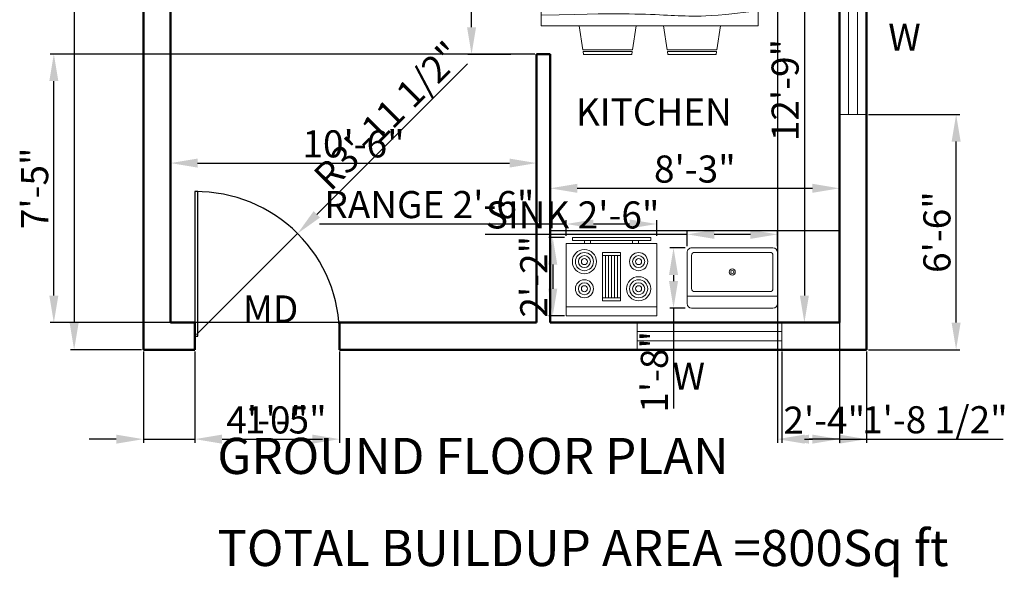
# Model space of a CAD drawing. Units: inches. Extents: x 1802 to 2621, y 1038 to 1686.
# Tile 1 of 5: x 1835 to 2161, y 1038 to 1223. Entities that reach past the tile are written whole.
import ezdxf

# ---------------------------------------------------------------- set-up
doc = ezdxf.new("R2010")
doc.units = ezdxf.units.IN
for name, color, linetype, lineweight in [('A-ANNO-DIMS', 2, 'Continuous', 18), ('A-ANNO-TEXT', 7, 'Continuous', 18), ('A-AREA-IDEN', 7, 'Continuous', 25), ('A-DOOR', 3, 'Continuous', 25), ('A-EQPM', 8, 'Continuous', 18), ('A-FLOR-CASE', 8, 'Continuous', 25), ('A-FLOR-FIXT', 9, 'Continuous', 18), ('A-FURN', 8, 'Continuous', 18), ('A-GLAZ', 4, 'Continuous', 18), ('A-WALL', 7, 'Continuous', 50)]:
    doc.layers.add(name, color=color, linetype=linetype, lineweight=lineweight)
doc.styles.get("Standard").update_dxf_attribs({"font": 'arial.ttf'})
doc.dimstyles.new('ISO-25', dxfattribs={"dimtxt": 9, "dimasz": 9, "dimexe": 1.25, "dimexo": 0.625, "dimtad": 1, "dimdec": 1, "dimrnd": 9, "dimlunit": 3, "dimtxsty": 'Standard', "dimcen": 2.5, "dimadec": 0, "dimazin": 0, "dimtfac": 1, "dimtdec": 1, "dimtmove": 0, "dimatfit": 3, "dimfxl": 1, "dimarcsym": 0})

# ---------------------------------------------------------------- blocks, each defined once
blk = doc.blocks.new('*D4')
at = {"layer": 'A-ANNO-DIMS', "color": 0, "lineweight": -2, "transparency": 16777216}
for p, q in [((1875.1, 1593.56), (1851.51, 1593.56)), ((1852.76, 1584.56), (1852.76, 1122.56)), ((1875.1, 1113.56), (1851.51, 1113.56))]:
    blk.add_line(p, q, dxfattribs=at)
at = {"layer": 'A-ANNO-DIMS', "color": 0, "transparency": 16777216}
for points in [[(1851.26, 1584.56), (1854.26, 1584.56), (1852.76, 1593.56)], [(1851.26, 1122.56), (1854.26, 1122.56), (1852.76, 1113.56)]]:
    blk.add_solid(points, dxfattribs=at)
at = {"layer": 'Defpoints', "color": 0, "transparency": 16777216}
for p in [(1875.73, 1593.56), (1852.76, 1113.56), (1875.73, 1113.56)]:
    blk.add_point(p, dxfattribs=at)
at = {"layer": 'A-ANNO-DIMS', "color": 0, "transparency": 16777216, "insert": (1847.54, 1353.56), "char_height": 9, "attachment_point": 5, "rotation": 90}
blk.add_mtext('39\'-9"', dxfattribs=at)
blk = doc.blocks.new('*D8')
at = {"layer": 'A-ANNO-DIMS', "color": 0, "lineweight": -2, "transparency": 16777216}
for p, q in [((2106.1, 1277.06), (2093.83, 1277.06)), ((2095.08, 1268.06), (2095.08, 1131.56)), ((2106.1, 1122.56), (2093.83, 1122.56))]:
    blk.add_line(p, q, dxfattribs=at)
at = {"layer": 'A-ANNO-DIMS', "color": 0, "transparency": 16777216}
for points in [[(2093.58, 1268.06), (2096.58, 1268.06), (2095.08, 1277.06)], [(2093.58, 1131.56), (2096.58, 1131.56), (2095.08, 1122.56)]]:
    blk.add_solid(points, dxfattribs=at)
at = {"layer": 'Defpoints', "color": 0, "transparency": 16777216}
for p in [(2106.73, 1277.06), (2095.08, 1122.56), (2106.73, 1122.56)]:
    blk.add_point(p, dxfattribs=at)
at = {"layer": 'A-ANNO-DIMS', "color": 0, "transparency": 16777216, "insert": (2089.86, 1199.81), "char_height": 9, "attachment_point": 5, "rotation": 90}
blk.add_mtext('12\'-9"', dxfattribs=at)
blk = doc.blocks.new('*D9')
at = {"layer": 'A-ANNO-DIMS', "color": 0, "lineweight": -2, "transparency": 16777216}
for p, q in [((2010.73, 1123.18), (2010.73, 1168.42)), ((2019.73, 1167.17), (2097.73, 1167.17)), ((2106.73, 1123.18), (2106.73, 1168.42))]:
    blk.add_line(p, q, dxfattribs=at)
at = {"layer": 'A-ANNO-DIMS', "color": 0, "transparency": 16777216}
for points in [[(2019.73, 1168.67), (2019.73, 1165.67), (2010.73, 1167.17)], [(2097.73, 1168.67), (2097.73, 1165.67), (2106.73, 1167.17)]]:
    blk.add_solid(points, dxfattribs=at)
at = {"layer": 'Defpoints', "color": 0, "transparency": 16777216}
for p in [(2106.73, 1167.17), (2010.73, 1122.56), (2106.73, 1122.56)]:
    blk.add_point(p, dxfattribs=at)
at = {"layer": 'A-ANNO-DIMS', "color": 0, "transparency": 16777216, "insert": (2058.73, 1172.4), "char_height": 9, "attachment_point": 5}
blk.add_mtext('8\'-3"', dxfattribs=at)
blk = doc.blocks.new('*D10')
at = {"layer": 'A-ANNO-DIMS', "color": 0, "lineweight": -2, "transparency": 16777216}
for p, q in [((1884.73, 1123.18), (1884.73, 1176.79)), ((2006.23, 1123.18), (2006.23, 1176.79)), ((1893.73, 1175.54), (1997.23, 1175.54))]:
    blk.add_line(p, q, dxfattribs=at)
at = {"layer": 'A-ANNO-DIMS', "color": 0, "transparency": 16777216}
for points in [[(1893.73, 1177.04), (1893.73, 1174.04), (1884.73, 1175.54)], [(1997.23, 1177.04), (1997.23, 1174.04), (2006.23, 1175.54)]]:
    blk.add_solid(points, dxfattribs=at)
at = {"layer": 'Defpoints', "color": 0, "transparency": 16777216}
for p in [(2006.23, 1175.54), (1884.73, 1122.56), (2006.23, 1122.56)]:
    blk.add_point(p, dxfattribs=at)
at = {"layer": 'A-ANNO-DIMS', "color": 0, "transparency": 16777216, "insert": (1945.48, 1180.76), "char_height": 9, "attachment_point": 5}
blk.add_mtext('10\'-6"', dxfattribs=at)
blk = doc.blocks.new('Dining Set - 36 x 72 in.')
for p, q in [((-22, 27.5), (-22.1562, 26.50042)), ((-5.8416, 26.5), (-22.1534, 26.5)), ((-22, 27.5), (-6, 27.5)), ((-5.8437, 26.49966), (-6, 27.5)), ((6, 27.5), (5.8438, 26.50042)), ((22.1584, 26.5), (5.8466, 26.5)), ((6, 27.5), (22, 27.5)), ((22.1563, 26.49966), (22, 27.5)), ((-22.2343, 26.00059), (-23.4847, 17.99762)), ((-22.2304, 26), (-5.7608, 26)), ((-4.5152, 17.99762), (-5.7655, 25.99926)), ((5.7657, 26.00059), (4.5153, 17.99762)), ((5.7696, 26), (22.2392, 26)), ((23.4848, 17.99762), (22.2345, 25.99926)), ((36, 18), (-36, 18)), ((-36, 18), (-36, -18)), ((36, -18), (36, 18)), ((-45.5, 8), (-44.5004, 8.15617)), ((-45.5, 8), (-45.5, -8)), ((-44.5, -8.15843), (-44.5, 8.15338)), ((-44.0006, 8.23428), (-35.9976, 9.48474)), ((-44, 8.23041), (-44, -8.23915)), ((44.0006, 8.23428), (35.9976, 9.48474)), ((44, 8.23041), (44, -8.23915)), ((44.5, -8.15843), (44.5, 8.15338)), ((45.5, 8), (44.5005, 8.15617)), ((45.5, 8), (45.5, -8)), ((-44.4997, -8.15631), (-45.5, -8)), ((-35.9976, -9.48476), (-43.9993, -8.2345)), ((35.9976, -9.48476), (43.9993, -8.2345)), ((44.4997, -8.15631), (45.5, -8)), ((-36, -18), (36, -18)), ((-22.2343, -26.0006), (-23.4847, -17.99762)), ((-4.5152, -17.99762), (-5.7655, -25.99928)), ((5.7657, -26.0006), (4.5153, -17.99762)), ((23.4848, -17.99762), (22.2345, -25.99928)), ((-22.2304, -26), (-5.7608, -26)), ((5.7696, -26), (22.2392, -26)), ((-22, -27.5), (-22.1562, -26.50044)), ((-5.8416, -26.5), (-22.1534, -26.5)), ((-22, -27.5), (-6, -27.5)), ((-5.8437, -26.49967), (-6, -27.5)), ((6, -27.5), (5.8438, -26.50044)), ((22.1584, -26.5), (5.8466, -26.5)), ((6, -27.5), (22, -27.5)), ((22.1563, -26.49967), (22, -27.5))]:
    blk.add_line(p, q)
for points in [[(-36, 15), (-31.1772, 14.97754), (-26.8079, 14.91406), (-22.8538, 14.81543), (-19.276, 14.6875), (-16.0362, 14.53613), (-13.0957, 14.36718), (-10.4159, 14.18652), (-7.9583, 14), (-5.6904, 13.81315), (-3.6035, 13.63021), (-1.6954, 13.45508), (0.0365, 13.29166), (1.5945, 13.14388), (2.9811, 13.01562), (4.1988, 12.9108), (5.25, 12.83333), (6.1393, 12.78613), (6.8802, 12.76823), (7.4883, 12.77767), (7.9792, 12.8125), (8.3685, 12.87077), (8.6719, 12.95052), (8.9049, 13.0498), (9.0833, 13.16666), (9.2205, 13.29899), (9.3216, 13.44401), (9.3895, 13.59879), (9.4271, 13.76041), (9.4373, 13.92594), (9.4232, 14.09245), (9.3875, 14.257), (9.3333, 14.41666), (9.2638, 14.56917), (9.1836, 14.71484), (9.0975, 14.85465), (9.0104, 14.98958), (8.9272, 15.1206), (8.8529, 15.2487), (8.7922, 15.37483), (8.75, 15.5), (8.7305, 15.62467), (8.7344, 15.74739), (8.7617, 15.86621), (8.8125, 15.97916), (8.8867, 16.08431), (8.9844, 16.17968), (9.1055, 16.26334), (9.25, 16.33333), (9.4189, 16.38802), (9.6172, 16.42708), (9.8506, 16.45052), (10.125, 16.45833), (10.4463, 16.45052), (10.8203, 16.42708), (11.2529, 16.38802), (11.75, 16.33333), (12.3184, 16.26318), (12.9694, 16.17838), (13.7151, 16.07991), (14.5677, 15.96875), (15.5395, 15.84586), (16.6426, 15.71224), (17.8893, 15.56884), (19.2917, 15.41666), (20.859, 15.25667), (22.5879, 15.08984), (24.4721, 14.91715), (26.5052, 14.73958), (28.6809, 14.5581), (30.9929, 14.3737), (33.4347, 14.18733), (36, 14)], [(-36, 10), (-28.9766, 10.14274), (-23.1725, 10.20442), (-18.4241, 10.19775), (-14.5677, 10.13541), (-11.4399, 10.03011), (-8.877, 9.89453), (-6.7154, 9.74137), (-4.7917, 9.58333), (-2.9698, 9.43082), (-1.2246, 9.28515), (0.4415, 9.14534), (2.026, 9.01041), (3.5266, 8.87939), (4.9408, 8.7513), (6.266, 8.62516), (7.5, 8.5), (8.6411, 8.37549), (9.6914, 8.2539), (10.6538, 8.13818), (11.5312, 8.03125), (12.3267, 7.93603), (13.043, 7.85547), (13.6831, 7.79248), (14.25, 7.75), (14.7471, 7.7303), (15.1797, 7.73307), (15.5537, 7.75732), (15.875, 7.80208), (16.1494, 7.86637), (16.3828, 7.94922), (16.5811, 8.04964), (16.75, 8.16666), (16.8944, 8.29915), (17.0143, 8.44531), (17.1089, 8.60319), (17.1771, 8.77083), (17.218, 8.94629), (17.2305, 9.1276), (17.2137, 9.31282), (17.1667, 9.5), (17.0895, 9.6875), (16.987, 9.875), (16.8649, 10.0625), (16.7292, 10.25), (16.5856, 10.4375), (16.4401, 10.625), (16.2985, 10.8125), (16.1667, 11), (16.05, 11.18733), (15.9518, 11.3737), (15.8752, 11.5581), (15.8229, 11.73958), (15.798, 11.91715), (15.8034, 12.08984), (15.842, 12.25667), (15.9167, 12.41666), (16.0295, 12.56836), (16.1784, 12.70833), (16.3605, 12.83268), (16.5729, 12.9375), (16.8127, 13.01888), (17.0768, 13.07291), (17.3625, 13.0957), (17.6667, 13.08333), (17.9894, 13.03312), (18.3418, 12.94726), (18.7382, 12.82918), (19.1927, 12.68229), (19.7195, 12.51001), (20.3327, 12.31575), (21.0465, 12.10294), (21.875, 11.875), (22.8357, 11.63354), (23.959, 11.37304), (25.2786, 11.08618), (26.8282, 10.76562), (28.6414, 10.40405), (30.752, 9.99414), (33.1936, 9.52856), (36, 9)], [(-36, 5.5), (-30.7157, 5.3348), (-26.069, 5.20963), (-21.9946, 5.11767), (-18.4271, 5.05208), (-15.3009, 5.00602), (-12.5508, 4.97265), (-10.1112, 4.94515), (-7.9167, 4.91666), (-5.909, 4.88167), (-4.0586, 4.83984), (-2.3429, 4.79215), (-0.7396, 4.73958), (0.7739, 4.6831), (2.22, 4.6237), (3.6213, 4.56233), (5, 4.5), (6.373, 4.43782), (7.7344, 4.3776), (9.0723, 4.32129), (10.375, 4.27083), (11.6309, 4.22819), (12.8281, 4.19531), (13.9551, 4.17415), (15, 4.16666), (15.954, 4.17448), (16.819, 4.19791), (17.6001, 4.23698), (18.3021, 4.29166), (18.9299, 4.36198), (19.4883, 4.44791), (19.9823, 4.54948), (20.4167, 4.66666), (20.7969, 4.79899), (21.1302, 4.94401), (21.4245, 5.09879), (21.6875, 5.26041), (21.9271, 5.42594), (22.1511, 5.59245), (22.3672, 5.757), (22.5834, 5.91666), (22.8065, 6.06868), (23.0404, 6.21093), (23.2879, 6.34147), (23.5521, 6.45833), (23.8358, 6.55957), (24.142, 6.64323), (24.4735, 6.70735), (24.8334, 6.75), (25.2235, 6.76969), (25.642, 6.76692), (26.0858, 6.74267), (26.5521, 6.69791), (27.0379, 6.63362), (27.5404, 6.55078), (28.0565, 6.45036), (28.5834, 6.33333), (29.1242, 6.19987), (29.7071, 6.04687), (30.3661, 5.87044), (31.1354, 5.66666), (32.0493, 5.43164), (33.142, 5.16146), (34.4475, 4.85221), (36, 4.5)], [(-36, -1), (-30.7915, -0.6591), (-26.0195, -0.38216), (-21.6519, -0.16284), (-17.6563, 0.00521), (-14.0005, 0.12833), (-10.6523, 0.21289), (-7.5796, 0.26522), (-4.75, 0.29166), (-2.134, 0.29793), (0.2878, 0.28711), (2.5317, 0.26163), (4.6146, 0.22396), (6.5529, 0.17651), (8.3633, 0.12174), (10.0623, 0.06209), (11.6667, 0), (13.1899, -0.06201), (14.6341, -0.1211), (15.9982, -0.17432), (17.2813, -0.21875), (18.4823, -0.25147), (19.6003, -0.26953), (20.6343, -0.27002), (21.5834, -0.25), (22.4481, -0.20768), (23.2357, -0.14584), (23.9549, -0.06836), (24.6146, 0.02083), (25.2235, 0.11784), (25.7904, 0.21875), (26.3241, 0.31966), (26.8334, 0.41666), (27.3265, 0.50618), (27.8099, 0.58593), (28.2894, 0.65397), (28.7709, 0.70833), (29.2601, 0.74707), (29.763, 0.76823), (30.2855, 0.76985), (30.8334, 0.75), (31.4088, 0.70784), (31.9994, 0.64713), (32.589, 0.57275), (33.1615, 0.48958), (33.7008, 0.4025), (34.1908, 0.3164), (34.6153, 0.23616), (34.9584, 0.16666), (35.2099, 0.11165), (35.3848, 0.07031), (35.504, 0.04069), (35.5886, 0.02083), (35.6594, 0.00879), (35.7377, 0.0026), (35.8442, 0.00032), (36, 0)], [(-36, -6.5), (-27.1843, -6.31267), (-20.084, -6.1263), (-14.469, -5.9419), (-10.1094, -5.76042), (-6.7752, -5.58285), (-4.2363, -5.41016), (-2.2629, -5.24333), (-0.625, -5.08334), (0.8708, -4.93099), (2.2715, -4.78646), (3.5872, -4.64974), (4.8281, -4.52084), (6.0046, -4.39974), (7.127, -4.28646), (8.2053, -4.18099), (9.25, -4.08334), (10.2705, -3.99382), (11.2734, -3.91407), (12.2647, -3.84603), (13.25, -3.79167), (14.2354, -3.75293), (15.2266, -3.73177), (16.2295, -3.73015), (17.25, -3.75), (18.2912, -3.79248), (19.3451, -3.85547), (20.4009, -3.93604), (21.4479, -4.03125), (22.4754, -4.13819), (23.4727, -4.25391), (24.4289, -4.37549), (25.3334, -4.5), (26.1785, -4.62492), (26.9694, -4.74935), (27.7145, -4.87281), (28.4219, -4.99479), (29.1, -5.11483), (29.7572, -5.23242), (30.4016, -5.34709), (31.0417, -5.45834), (31.6837, -5.56437), (32.3262, -5.65821), (32.9658, -5.73153), (33.599, -5.77604), (34.2224, -5.78345), (34.8327, -5.74545), (35.4264, -5.65373), (36, -5.5)], [(-36, -10), (-26.4022, -9.81299), (-18.4675, -9.62891), (-11.9839, -9.45069), (-6.7396, -9.28125), (-2.5226, -9.12354), (0.8789, -8.98047), (3.6769, -8.85498), (6.0833, -8.75), (8.2767, -8.66765), (10.3021, -8.60677), (12.1712, -8.56543), (13.8958, -8.54167), (15.4876, -8.53353), (16.9583, -8.53907), (18.3197, -8.55632), (19.5834, -8.58334), (20.7616, -8.61841), (21.8685, -8.66081), (22.9188, -8.71004), (23.9271, -8.76563), (24.9081, -8.82707), (25.8763, -8.89388), (26.8465, -8.96558), (27.8334, -9.04167), (28.8474, -9.12118), (29.8828, -9.20117), (30.93, -9.27824), (31.9792, -9.34896), (33.0205, -9.40991), (34.0443, -9.45768), (35.0407, -9.48885), (36, -9.5)], [(-36, -14.5), (-30.0881, -14.33513), (-25.0332, -14.21224), (-20.7312, -14.12647), (-17.0781, -14.07292), (-13.97, -14.04671), (-11.3027, -14.04297), (-8.9724, -14.05681), (-6.875, -14.08334), (-4.9224, -14.11833), (-3.0905, -14.16016), (-1.3709, -14.20785), (0.2448, -14.26042), (1.7647, -14.3169), (3.1973, -14.3763), (4.5507, -14.43767), (5.8333, -14.5), (7.0554, -14.5621), (8.235, -14.62175), (9.3922, -14.67652), (10.5469, -14.72396), (11.7192, -14.76164), (12.929, -14.78711), (14.1965, -14.79794), (15.5417, -14.79167), (16.9933, -14.76424), (18.6152, -14.70508), (20.4804, -14.60197), (22.6615, -14.44271), (25.2312, -14.21509), (28.2624, -13.9069), (31.8277, -13.50594), (36, -13)]]:
    blk.add_lwpolyline(points)
blk = doc.blocks.new('Range-Oven - 30 in top')
for p, q in [((0, -3), (30, -3)), ((12, -6), (18, -6)), ((13, -20), (13, -6)), ((14, -6), (14, -20)), ((15, -20), (15, -6)), ((16, -6), (16, -20)), ((17, -20), (17, -6)), ((18, -20), (12, -20)), ((6, -24), (6, -25)), ((8, -25), (8, -24)), ((22, -25), (22, -24)), ((24, -24), (24, -25))]:
    blk.add_line(p, q)
for points in [[(0, -24), (0, 0), (30, 0), (30, -24)], [(12, -21), (12, -5), (18, -5), (18, -21)], [(2, -26), (2, -25), (28, -25), (28, -26)]]:
    blk.add_lwpolyline(points, close=True)
for centre, radius in [((6, -9), 4), ((6, -9), 3), ((24, -9), 3), ((6, -9), 2), ((6, -9), 1), ((24, -9), 2), ((24, -9), 1), ((6, -18), 3), ((6, -18), 2), ((24, -18), 4), ((24, -18), 3), ((24, -18), 2), ((6, -18), 1), ((24, -18), 1)]:
    blk.add_circle(centre, radius)
blk = doc.blocks.new('Sink-single - 30 in top')
blk.add_line((-15, -3.999996), (15, -3.999996))
for points in [[(-13.5, 0), (13.5, 0)], [(-15, -18.499996), (-15, -1.5)], [(15, -1.5), (15, -18.499996)], [(-13.5, -17.499996), (-13.5, -6.499996)], [(-12.5, -5.499996), (12.5, -5.499996)], [(13.5, -6.499996), (13.5, -17.499996)], [(12.5, -18.499996), (-12.5, -18.499996)], [(13.5, -19.999996), (-13.5, -19.999996)]]:
    blk.add_lwpolyline(points)
for radius in [1, 0.5]:
    blk.add_circle((0, -11.999996), radius)
for centre, radius, start, end in [((-13.5, -1.5), 1.5, 90, 180), ((13.5, -1.5), 1.5, 0, 90), ((-12.5, -6.499996), 1, 90, 180), ((12.5, -6.499996), 1, 0, 90), ((-13.5, -18.499996), 1.5, 180, 270), ((-12.5, -17.499996), 1, 180, 270), ((12.5, -17.499996), 1, 270, 0), ((13.5, -18.499996), 1.5, 270, 0)]:
    blk.add_arc(centre, radius, start, end)
blk = doc.blocks.new('WIN-48IN')
for p, q in [((9, 48), (0, 48)), ((3, 48), (3, 0)), ((6, 48), (6, 0)), ((9, 0), (0, 0))]:
    blk.add_line(p, q)
blk = doc.blocks.new('*D60')
at = {"layer": 'A-ANNO-DIMS', "color": 0, "lineweight": -2, "transparency": 16777216}
for p, q in [((1997.66, 1266.65), (1983.38, 1266.65)), ((1984.63, 1220.65), (1984.63, 1257.65)), ((1997.66, 1211.65), (1983.38, 1211.65))]:
    blk.add_line(p, q, dxfattribs=at)
at = {"layer": 'A-ANNO-DIMS', "color": 0, "transparency": 16777216}
for points in [[(1983.13, 1257.65), (1986.13, 1257.65), (1984.63, 1266.65)], [(1983.13, 1220.65), (1986.13, 1220.65), (1984.63, 1211.65)]]:
    blk.add_solid(points, dxfattribs=at)
at = {"layer": 'Defpoints', "color": 0, "transparency": 16777216}
for p in [(1984.63, 1266.65), (1998.28, 1266.65), (1998.28, 1211.65)]:
    blk.add_point(p, dxfattribs=at)
at = {"layer": 'A-ANNO-DIMS', "color": 0, "transparency": 16777216, "insert": (1979.51, 1239.15), "char_height": 9, "attachment_point": 5, "rotation": 90}
blk.add_mtext('4\'-7"', dxfattribs=at)
blk = doc.blocks.new('*D61')
at = {"layer": 'A-ANNO-DIMS', "color": 0, "lineweight": -2, "transparency": 16777216}
for p, q in [((2016.08, 1155.31), (1934.17, 1155.31)), ((2016.08, 1151.43), (2016.08, 1156.56)), ((2037.08, 1155.31), (2025.08, 1155.31)), ((2046.08, 1151.43), (2046.08, 1156.56))]:
    blk.add_line(p, q, dxfattribs=at)
at = {"layer": 'A-ANNO-DIMS', "color": 0, "transparency": 16777216}
for points in [[(2025.08, 1156.81), (2025.08, 1153.81), (2016.08, 1155.31)], [(2037.08, 1156.81), (2037.08, 1153.81), (2046.08, 1155.31)]]:
    blk.add_solid(points, dxfattribs=at)
at = {"layer": 'Defpoints', "color": 0, "transparency": 16777216}
for p in [(2016.08, 1155.31), (2016.08, 1150.81), (2046.08, 1150.81)]:
    blk.add_point(p, dxfattribs=at)
at = {"layer": 'A-ANNO-DIMS', "color": 0, "transparency": 16777216, "insert": (1970.63, 1160.59), "char_height": 9, "attachment_point": 5}
blk.add_mtext('RANGE 2\'-6"', dxfattribs=at)
blk = doc.blocks.new('*D62')
at = {"layer": 'A-ANNO-DIMS', "color": 0, "lineweight": -2, "transparency": 16777216}
for p, q in [((2015.46, 1150.81), (2010.33, 1150.81)), ((2011.58, 1141.81), (2011.58, 1133.81)), ((2015.46, 1124.81), (2010.33, 1124.81))]:
    blk.add_line(p, q, dxfattribs=at)
at = {"layer": 'A-ANNO-DIMS', "color": 0, "transparency": 16777216}
for points in [[(2010.08, 1141.81), (2013.08, 1141.81), (2011.58, 1150.81)], [(2010.08, 1133.81), (2013.08, 1133.81), (2011.58, 1124.81)]]:
    blk.add_solid(points, dxfattribs=at)
at = {"layer": 'Defpoints', "color": 0, "transparency": 16777216}
for p in [(2016.08, 1150.81), (2011.58, 1124.81), (2016.08, 1124.81)]:
    blk.add_point(p, dxfattribs=at)
at = {"layer": 'A-ANNO-DIMS', "color": 0, "transparency": 16777216, "insert": (2006.44, 1137.81), "char_height": 9, "attachment_point": 5, "rotation": 90}
blk.add_mtext('2\'-2"', dxfattribs=at)
blk = doc.blocks.new('*D63')
at = {"layer": 'A-ANNO-DIMS', "color": 0, "lineweight": -2, "transparency": 16777216}
for p, q in [((2056.16, 1151.87), (1989.19, 1151.87)), ((2056.16, 1148), (2056.16, 1153.12)), ((2077.16, 1151.87), (2065.16, 1151.87)), ((2086.16, 1148), (2086.16, 1153.12))]:
    blk.add_line(p, q, dxfattribs=at)
at = {"layer": 'A-ANNO-DIMS', "color": 0, "transparency": 16777216}
for points in [[(2065.16, 1153.37), (2065.16, 1150.37), (2056.16, 1151.87)], [(2077.16, 1153.37), (2077.16, 1150.37), (2086.16, 1151.87)]]:
    blk.add_solid(points, dxfattribs=at)
at = {"layer": 'Defpoints', "color": 0, "transparency": 16777216}
for p in [(2056.16, 1151.87), (2056.16, 1147.37), (2086.16, 1147.37)]:
    blk.add_point(p, dxfattribs=at)
at = {"layer": 'A-ANNO-DIMS', "color": 0, "transparency": 16777216, "insert": (2018.18, 1157.15), "char_height": 9, "attachment_point": 5}
blk.add_mtext('SINK 2\'-6"', dxfattribs=at)
blk = doc.blocks.new('*D64')
at = {"layer": 'A-ANNO-DIMS', "color": 0, "lineweight": -2, "transparency": 16777216}
for p, q in [((2055.54, 1147.37), (2050.41, 1147.37)), ((2051.66, 1138.37), (2051.66, 1136.37)), ((2055.54, 1127.37), (2050.41, 1127.37)), ((2051.66, 1127.37), (2051.66, 1094.05))]:
    blk.add_line(p, q, dxfattribs=at)
at = {"layer": 'A-ANNO-DIMS', "color": 0, "transparency": 16777216}
for points in [[(2050.16, 1138.37), (2053.16, 1138.37), (2051.66, 1147.37)], [(2050.16, 1136.37), (2053.16, 1136.37), (2051.66, 1127.37)]]:
    blk.add_solid(points, dxfattribs=at)
at = {"layer": 'Defpoints', "color": 0, "transparency": 16777216}
for p in [(2056.16, 1147.37), (2051.66, 1127.37), (2056.16, 1127.37)]:
    blk.add_point(p, dxfattribs=at)
at = {"layer": 'A-ANNO-DIMS', "color": 0, "transparency": 16777216, "insert": (2046.44, 1106.21), "char_height": 9, "attachment_point": 5, "rotation": 90}
blk.add_mtext('1\'-8"', dxfattribs=at)
blk = doc.blocks.new('*D65')
at = {"layer": 'A-ANNO-DIMS', "color": 0, "lineweight": -2, "transparency": 16777216}
for p, q in [((1875.73, 1112.93), (1875.73, 1082.61)), ((1892.83, 1112.93), (1892.83, 1082.61)), ((1866.73, 1083.86), (1857.73, 1083.86)), ((1875.73, 1083.86), (1892.83, 1083.86)), ((1901.83, 1083.86), (1935.16, 1083.86))]:
    blk.add_line(p, q, dxfattribs=at)
at = {"layer": 'A-ANNO-DIMS', "color": 0, "transparency": 16777216}
for points in [[(1866.73, 1085.36), (1866.73, 1082.36), (1875.73, 1083.86)], [(1901.83, 1085.36), (1901.83, 1082.36), (1892.83, 1083.86)]]:
    blk.add_solid(points, dxfattribs=at)
at = {"layer": 'Defpoints', "color": 0, "transparency": 16777216}
for p in [(1875.73, 1113.56), (1892.83, 1113.56), (1892.83, 1083.86)]:
    blk.add_point(p, dxfattribs=at)
at = {"layer": 'A-ANNO-DIMS', "color": 0, "transparency": 16777216, "insert": (1922.99, 1089.08), "char_height": 9, "attachment_point": 5}
blk.add_mtext('1\'-5"', dxfattribs=at)
blk = doc.blocks.new('*D72')
at = {"layer": 'A-ANNO-DIMS', "color": 0, "lineweight": -2, "transparency": 16777216}
for p, q in [((2116.35, 1191.68), (2146.68, 1191.68)), ((2145.43, 1122.56), (2145.43, 1182.68)), ((2116.35, 1113.56), (2146.68, 1113.56))]:
    blk.add_line(p, q, dxfattribs=at)
at = {"layer": 'A-ANNO-DIMS', "color": 0, "transparency": 16777216}
for points in [[(2143.93, 1182.68), (2146.93, 1182.68), (2145.43, 1191.68)], [(2143.93, 1122.56), (2146.93, 1122.56), (2145.43, 1113.56)]]:
    blk.add_solid(points, dxfattribs=at)
at = {"layer": 'Defpoints', "color": 0, "transparency": 16777216}
for p in [(2115.73, 1191.68), (2145.43, 1191.68), (2115.73, 1113.56)]:
    blk.add_point(p, dxfattribs=at)
at = {"layer": 'A-ANNO-DIMS', "color": 0, "transparency": 16777216, "insert": (2140.21, 1152.62), "char_height": 9, "attachment_point": 5, "rotation": 90}
blk.add_mtext('6\'-6"', dxfattribs=at)
blk = doc.blocks.new('*D73')
at = {"layer": 'A-ANNO-DIMS', "color": 0, "lineweight": -2, "transparency": 16777216}
for p, q in [((2087.63, 1112.93), (2087.63, 1082.61)), ((2115.73, 1112.93), (2115.73, 1082.61)), ((2106.73, 1083.86), (2096.63, 1083.86))]:
    blk.add_line(p, q, dxfattribs=at)
at = {"layer": 'A-ANNO-DIMS', "color": 0, "transparency": 16777216}
for points in [[(2096.63, 1085.36), (2096.63, 1082.36), (2087.63, 1083.86)], [(2106.73, 1085.36), (2106.73, 1082.36), (2115.73, 1083.86)]]:
    blk.add_solid(points, dxfattribs=at)
at = {"layer": 'Defpoints', "color": 0, "transparency": 16777216}
for p in [(2087.63, 1113.56), (2115.73, 1113.56), (2087.63, 1083.86)]:
    blk.add_point(p, dxfattribs=at)
at = {"layer": 'A-ANNO-DIMS', "color": 0, "transparency": 16777216, "insert": (2101.68, 1089), "char_height": 9, "attachment_point": 5}
blk.add_mtext('2\'-4"', dxfattribs=at)
blk = doc.blocks.new('*D74')
at = {"layer": 'A-ANNO-DIMS', "color": 0, "lineweight": -2, "transparency": 16777216}
for p, q in [((1892.83, 1112.93), (1892.83, 1082.61)), ((1940.83, 1112.93), (1940.83, 1082.61)), ((1901.83, 1083.86), (1931.83, 1083.86))]:
    blk.add_line(p, q, dxfattribs=at)
at = {"layer": 'A-ANNO-DIMS', "color": 0, "transparency": 16777216}
for points in [[(1901.83, 1085.36), (1901.83, 1082.36), (1892.83, 1083.86)], [(1931.83, 1085.36), (1931.83, 1082.36), (1940.83, 1083.86)]]:
    blk.add_solid(points, dxfattribs=at)
at = {"layer": 'Defpoints', "color": 0, "transparency": 16777216}
for p in [(1892.83, 1113.56), (1940.83, 1113.56), (1940.83, 1083.86)]:
    blk.add_point(p, dxfattribs=at)
at = {"layer": 'A-ANNO-DIMS', "color": 0, "transparency": 16777216, "insert": (1916.83, 1089.08), "char_height": 9, "attachment_point": 5}
blk.add_mtext('4\'-0"', dxfattribs=at)
blk = doc.blocks.new('*D75')
at = {"layer": 'A-ANNO-DIMS', "color": 0, "lineweight": -2, "transparency": 16777216}
for p, q in [((2086.14, 1280.93), (2086.14, 1082.61)), ((2106.73, 1278.98), (2106.73, 1082.61)), ((2095.14, 1083.86), (2097.73, 1083.86)), ((2106.73, 1083.86), (2161.03, 1083.86))]:
    blk.add_line(p, q, dxfattribs=at)
at = {"layer": 'A-ANNO-DIMS', "color": 0, "transparency": 16777216}
for points in [[(2095.14, 1085.36), (2095.14, 1082.36), (2086.14, 1083.86)], [(2097.73, 1085.36), (2097.73, 1082.36), (2106.73, 1083.86)]]:
    blk.add_solid(points, dxfattribs=at)
at = {"layer": 'Defpoints', "color": 0, "transparency": 16777216}
for p in [(2086.14, 1281.56), (2106.73, 1279.61), (2106.73, 1083.86)]:
    blk.add_point(p, dxfattribs=at)
at = {"layer": 'A-ANNO-DIMS', "color": 0, "transparency": 16777216, "insert": (2138.38, 1089.14), "char_height": 9, "attachment_point": 5}
blk.add_mtext('1\'-8 1/2"', dxfattribs=at)
blk = doc.blocks.new('*D77')
at = {"layer": 'A-ANNO-DIMS', "color": 0, "lineweight": -2, "transparency": 16777216}
for p, q in [((2005.6, 1211.75), (1844.78, 1211.75)), ((1846.03, 1131.56), (1846.03, 1202.75)), ((2005.6, 1122.56), (1844.78, 1122.56))]:
    blk.add_line(p, q, dxfattribs=at)
at = {"layer": 'A-ANNO-DIMS', "color": 0, "transparency": 16777216}
for points in [[(1844.53, 1202.75), (1847.53, 1202.75), (1846.03, 1211.75)], [(1844.53, 1131.56), (1847.53, 1131.56), (1846.03, 1122.56)]]:
    blk.add_solid(points, dxfattribs=at)
at = {"layer": 'Defpoints', "color": 0, "transparency": 16777216}
for p in [(1846.03, 1211.75), (2006.23, 1211.75), (2006.23, 1122.56)]:
    blk.add_point(p, dxfattribs=at)
at = {"layer": 'A-ANNO-DIMS', "color": 0, "transparency": 16777216, "insert": (1840.83, 1167.15), "char_height": 9, "attachment_point": 5, "rotation": 90}
blk.add_mtext('7\'-5"', dxfattribs=at)
blk = doc.blocks.new('*D78')
at = {"layer": 'A-ANNO-DIMS', "color": 0, "lineweight": -2, "transparency": 16777216}
for p, q in [((1983.31, 1208.54), (1933.28, 1158.51)), ((1893.33, 1118.56), (1926.92, 1152.15))]:
    blk.add_line(p, q, dxfattribs=at)
at = {"layer": 'A-ANNO-DIMS', "color": 0, "transparency": 16777216}
blk.add_solid([(1932.22, 1159.57), (1934.34, 1157.45), (1926.92, 1152.15)], dxfattribs=at)
at = {"layer": 'Defpoints', "color": 0, "transparency": 16777216}
for p in [(1926.92, 1152.15), (1893.33, 1118.56)]:
    blk.add_point(p, dxfattribs=at)
at = {"layer": 'A-ANNO-DIMS', "color": 0, "transparency": 16777216, "insert": (1957.74, 1190.44), "char_height": 9, "attachment_point": 5, "rotation": 45}
blk.add_mtext('R3\'-11 1/2"', dxfattribs=at)

msp = doc.modelspace()

# ---------------------------------------------------------------- linework, layer by layer
at = {"layer": 'A-DOOR'}
for p, q in [((1893.83, 1166.06), (1892.83, 1166.06)), ((1892.83, 1166.06), (1892.83, 1122.56)), ((1893.83, 1118.06), (1893.83, 1166.06)), ((1892.83, 1118.06), (1893.83, 1118.06))]:
    msp.add_line(p, q, dxfattribs=at)
msp.add_arc((1893.33, 1118.56), 47.5, 359.3969, 90.6031, dxfattribs=at)
at = {"layer": 'A-FLOR-CASE'}
msp.add_line((2010.73, 1153.18), (2106.73, 1153.18), dxfattribs=at)
at = {"layer": 'A-WALL'}
for p, q in [((1875.73, 1593.56), (1875.73, 1113.56)), ((2115.73, 1113.56), (2115.73, 1593.56)), ((1884.73, 1341.56), (1884.73, 1122.56)), ((2106.73, 1122.56), (2106.73, 1341.56)), ((2006.23, 1122.56), (2006.23, 1211.75)), ((2010.73, 1211.75), (2006.23, 1211.75)), ((2010.73, 1122.56), (2010.73, 1211.75)), ((1884.73, 1122.56), (1892.83, 1122.56)), ((1892.83, 1122.56), (1892.83, 1113.56)), ((1940.83, 1122.56), (1940.83, 1113.56)), ((1940.83, 1122.56), (2006.23, 1122.56)), ((2010.73, 1122.56), (2106.73, 1122.56)), ((1875.73, 1113.56), (1892.83, 1113.56)), ((1940.83, 1113.56), (2115.73, 1113.56))]:
    msp.add_line(p, q, dxfattribs=at)

# ---------------------------------------------------------------- block references
at = {"layer": 'A-EQPM', "rotation": 180}
msp.add_blockref('Range-Oven - 30 in top', (2046.08, 1124.81), dxfattribs=at)
at = {"layer": 'A-FLOR-FIXT', "rotation": 180}
msp.add_blockref('Sink-single - 30 in top', (2071.16, 1127.37), dxfattribs=at)
at = {"layer": 'A-FURN'}
msp.add_blockref('Dining Set - 36 x 72 in.', (2043.78, 1239.15), dxfattribs=at)
at = {"layer": 'A-GLAZ'}
for p, rotation in [((2115.73, 1239.68), 180), ((2039.63, 1122.56), 270.0000000000002)]:
    msp.add_blockref('WIN-48IN', p, dxfattribs=dict(at, rotation=rotation))

# ---------------------------------------------------------------- texts
at = {"layer": 'A-ANNO-TEXT', "attachment_point": 1}
for s, width, insert, char_height in [('W', 30.0361, (2122.91, 1221.84), 9), ('MD ', 17.1074, (1908.74, 1131.6), 9), ('W', 30.0361, (2051.33, 1109.3), 9), ('GROUND FLOOR PLAN', 217.7869, (1900.28, 1084.29), 12)]:
    msp.add_mtext_dynamic_manual_height_columns(s, width=width, gutter_width=12.5, heights=[0], dxfattribs=dict(at, insert=insert, char_height=char_height))
at = {"layer": 'A-AREA-IDEN', "attachment_point": 1}
for s, width, insert, char_height in [('KITCHEN', 82.6611, (2019.24, 1197.01), 9), ('TOTAL BUILDUP AREA =800Sq ft', 272.6952, (1900.28, 1053.72), 12)]:
    msp.add_mtext_dynamic_manual_height_columns(s, width=width, gutter_width=12.5, heights=[0], dxfattribs=dict(at, insert=insert, char_height=char_height))

# ---------------------------------------------------------------- dimensions: what is measured, and where the dimension line sits
at = {"layer": 'A-ANNO-DIMS'}
for base, p1, p2, angle, override, picture, middle in [((1852.76, 1113.56), (1875.73, 1593.56), (1875.73, 1113.56), 90, {"dimclrd": 0, "dimclre": 0, "dimclrt": 0}, '*D4', (1847.54, 1353.56)), ((2095.08, 1122.56), (2106.73, 1277.06), (2106.73, 1122.56), 90, {"dimclrd": 0, "dimclre": 0, "dimclrt": 0}, '*D8', (2089.86, 1199.81)), ((1984.63, 1266.65), (1998.28, 1211.65), (1998.28, 1266.65), 90, {"dimdec": 1, "dimlfac": 1, "dimrnd": 0, "dimzin": 1, "dimdsep": 46, "dimlunit": 4, "dimfrac": 2}, '*D60', (1979.51, 1239.15)), ((1846.03, 1211.75), (2006.23, 1122.56), (2006.23, 1211.75), 90, {"dimdec": 1, "dimlfac": 1, "dimrnd": 0, "dimzin": 1, "dimdsep": 46, "dimlunit": 4, "dimfrac": 2}, '*D77', (1840.83, 1167.15)), ((2145.43, 1191.68), (2115.73, 1113.56), (2115.73, 1191.68), 90, {"dimdec": 1, "dimlfac": 1, "dimrnd": 0, "dimzin": 1, "dimdsep": 46, "dimlunit": 4, "dimfrac": 2}, '*D72', (2140.21, 1152.62)), ((2011.58, 1124.81), (2016.08, 1150.81), (2016.08, 1124.81), 270, {"dimdec": 1, "dimlfac": 1, "dimrnd": 0, "dimzin": 1, "dimdsep": 46, "dimlunit": 4, "dimfrac": 2}, '*D62', (2006.44, 1137.81)), ((2051.66, 1127.37), (2056.16, 1147.37), (2056.16, 1127.37), 270, {"dimdec": 1, "dimlfac": 1, "dimrnd": 0, "dimzin": 1, "dimdsep": 46, "dimlunit": 4, "dimfrac": 2}, '*D64', (2046.44, 1106.21))]:
    dim = msp.add_linear_dim(base=base, p1=p1, p2=p2, angle=angle, dimstyle='ISO-25', override=override, dxfattribs=at)
    dim.commit()
    dim.dimension.update_dxf_attribs({"geometry": picture, "text_midpoint": middle})
for base, p1, p2, override, picture, middle in [((2106.73, 1083.86), (2086.14, 1281.56), (2106.73, 1279.61), {"dimdec": 1, "dimlfac": 1, "dimrnd": 0, "dimzin": 1, "dimdsep": 46, "dimlunit": 4, "dimfrac": 2}, '*D75', (2138.38, 1089.14)), ((2006.23, 1175.54), (1884.73, 1122.56), (2006.23, 1122.56), {"dimclrd": 0, "dimclre": 0, "dimclrt": 0}, '*D10', (1945.48, 1180.76)), ((2106.73, 1167.17), (2010.73, 1122.56), (2106.73, 1122.56), {"dimclrd": 0, "dimclre": 0, "dimclrt": 0}, '*D9', (2058.73, 1172.4)), ((1892.83, 1083.86), (1875.73, 1113.56), (1892.83, 1113.56), {"dimdec": 1, "dimlfac": 1, "dimrnd": 0, "dimzin": 1, "dimdsep": 46, "dimlunit": 4, "dimfrac": 2}, '*D65', (1922.99, 1089.08)), ((1940.83, 1083.86), (1892.83, 1113.56), (1940.83, 1113.56), {"dimdec": 1, "dimlfac": 1, "dimrnd": 0, "dimzin": 1, "dimdsep": 46, "dimlunit": 4, "dimfrac": 2}, '*D74', (1916.83, 1089.08)), ((2087.63, 1083.86), (2115.73, 1113.56), (2087.63, 1113.56), {"dimdec": 1, "dimlfac": 1, "dimrnd": 0, "dimzin": 1, "dimdsep": 46, "dimlunit": 4, "dimfrac": 2}, '*D73', (2101.68, 1089))]:
    dim = msp.add_linear_dim(base=base, p1=p1, p2=p2, dimstyle='ISO-25', override=override, dxfattribs=at)
    dim.commit()
    dim.dimension.update_dxf_attribs({"geometry": picture, "text_midpoint": middle})
dim = msp.add_radius_dim(center=(1893.33, 1118.56), mpoint=(1926.92, 1152.15), dimstyle='ISO-25', override={"dimdec": 1, "dimlfac": 1, "dimrnd": 0, "dimzin": 1, "dimdsep": 46, "dimlunit": 4, "dimfrac": 2}, dxfattribs=at)
dim.commit()
dim.dimension.update_dxf_attribs({"geometry": '*D78', "text_midpoint": (1957.74, 1190.44)})
for base, p1, p2, text, picture, middle in [((2016.08, 1155.31), (2046.08, 1150.81), (2016.08, 1150.81), 'RANGE <>', '*D61', (1970.63, 1160.59)), ((2056.16, 1151.87), (2086.16, 1147.37), (2056.16, 1147.37), 'SINK <>', '*D63', (2018.18, 1157.15))]:
    dim = msp.add_linear_dim(base=base, p1=p1, p2=p2, angle=180, text=text, dimstyle='ISO-25', override={"dimdec": 1, "dimlfac": 1, "dimrnd": 0, "dimzin": 1, "dimdsep": 46, "dimlunit": 4, "dimfrac": 2}, dxfattribs=at)
    dim.commit()
    dim.dimension.update_dxf_attribs({"geometry": picture, "text_midpoint": middle})

doc.saveas('drawing.dxf')
